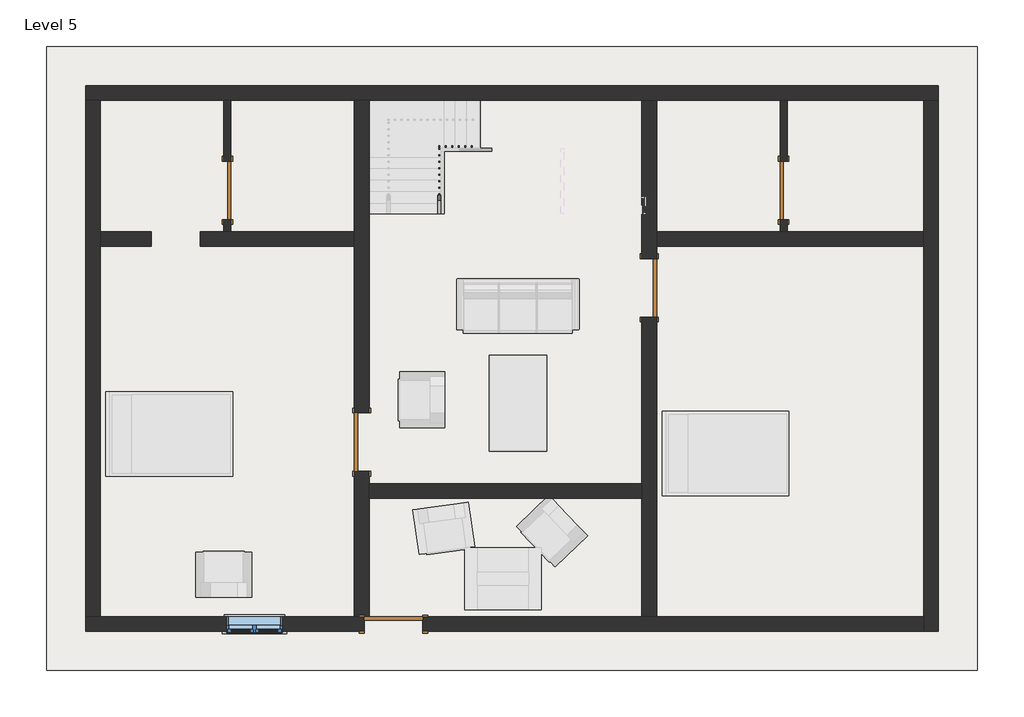
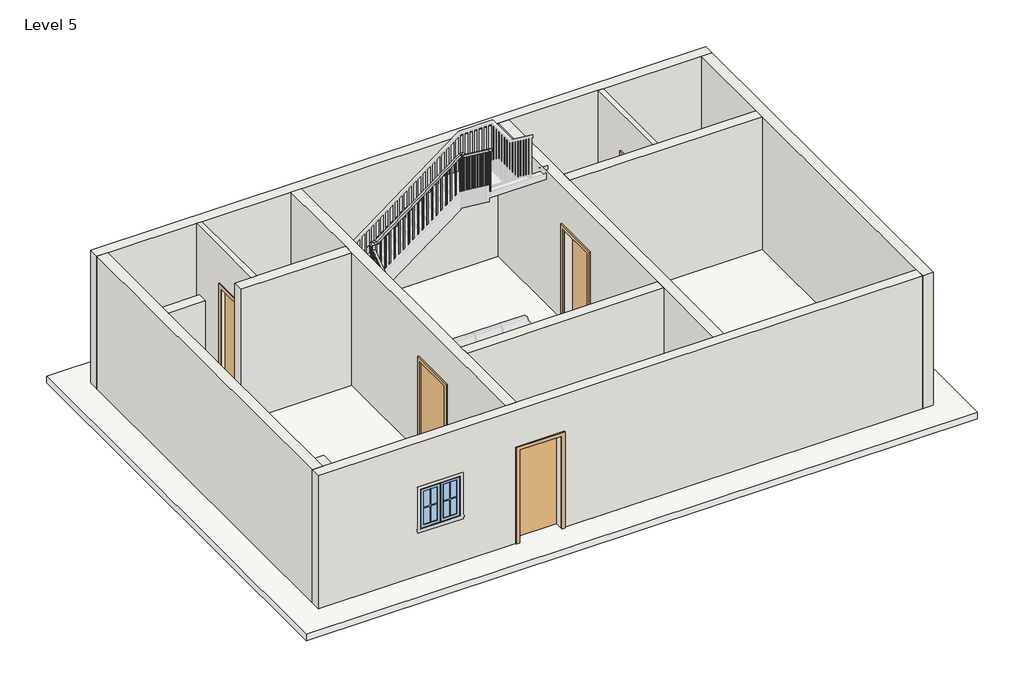
# One storey, part 1 of 2: 12 walls, 5 doors, 1 railing, 1 roof, 1 window.
"""IFC4 building model written with IfcOpenShell, lengths in millimetres."""

from ifc_helpers import new_model, si_unit, frame, origin, place, context, project, spatial, polyline, outline, extrude, faceted_brep, transform, mapped, element, save
from components import door_e5f9f3c4, door_a90ba1ad, door_305aa2a5, window_339605e1

model = new_model("IFC4")

# Units and contexts
model_context = context("Model", 3, world=origin())
ifc_project = project(units=[si_unit("LENGTHUNIT", "METRE", prefix="MILLI")], contexts=[model_context])

# Site, building, storey
site = spatial("IfcSite", under=ifc_project)
building = spatial("IfcBuilding", under=site)
storey = spatial("IfcBuildingStorey", under=building, Name="Level 5", Elevation=9601.2)

# Doors
placement = place(None, origin())
door_shape = door_e5f9f3c4(model_context)
element("IfcDoor", 1, ObjectType="Single-Flush : 36\" x 84\"", at=placement, inside=storey, context=model_context, shape_type="MappedRepresentation", body=[
    mapped(door_shape, transform((-5709.1546642, 5087.2167606, 9601.2), x_axis=(0.0, -1.0, 0.0), y_axis=(1.0, 0.0, 0.0), z_axis=(0.0, 0.0, 1.0))),
])
door_2_shape = door_a90ba1ad(model_context)
element("IfcDoor", 2, ObjectType="Single-Flush : 36\" x 84\"", at=placement, inside=storey, context=model_context, shape_type="MappedRepresentation", body=[
    mapped(door_2_shape, transform((-3607.3046642, 1150.2167606, 9601.2), x_axis=(0.0, -1.0, 0.0), y_axis=(1.0, 0.0, 0.0), z_axis=(0.0, 0.0, 1.0))),
])
element("IfcDoor", 3, ObjectType="Single-Flush : 36\" x 84\"", at=placement, inside=storey, context=model_context, shape_type="MappedRepresentation", body=[
    mapped(door_2_shape, transform((888.4953358, 3563.2167606, 9601.2), x_axis=(0.0, 1.0, 0.0), y_axis=(-1.0, 0.0, 0.0), z_axis=(0.0, 0.0, 1.0))),
])
element("IfcDoor", 4, ObjectType="Single-Flush : 36\" x 84\"", at=placement, inside=storey, context=model_context, shape_type="MappedRepresentation", body=[
    mapped(door_2_shape, transform((-3112.0046642, -1694.5832394, 9601.2), x_axis=(-1.0, 0.0, 0.0), y_axis=(0.0, -1.0, 0.0), z_axis=(0.0, 0.0, 1.0))),
])
door_3_shape = door_305aa2a5(model_context)
element("IfcDoor", 5, ObjectType="Single-Flush : 36\" x 84\"", at=placement, inside=storey, context=model_context, shape_type="MappedRepresentation", body=[
    mapped(door_3_shape, transform((2990.3453358, 5087.2167606, 9601.2), x_axis=(0.0, -1.0, 0.0), y_axis=(1.0, 0.0, 0.0), z_axis=(0.0, 0.0, 1.0))),
])

# Railing
element("IfcRailing", 6, ObjectType="Handrail - Rectangular", at=placement, inside=storey, context=model_context, shape_type="SolidModel", body=[
    faceted_brep([(-2419.4972892, 4718.9167606, 10648.1217391), (-2419.4972892, 4718.9167606, 10584.7634439), (-2368.6972892, 4718.9167606, 10584.7634439), (-2368.6972892, 4718.9167606, 10648.1217391), (-2419.4972892, 5670.3536537, 11357.2672495), (-2419.4972892, 5721.1536537, 11331.7723083), (-2368.6972892, 5721.1536537, 11331.7723083), (-2368.6972892, 5670.3536537, 11357.2672495), (-2419.4972892, 5670.3536537, 11464.0733611), (-2419.4972892, 5721.1536537, 11413.2733611), (-2368.6972892, 5721.1536537, 11413.2733611), (-2368.6972892, 5670.3536537, 11464.0733611), (-2419.4972892, 5797.3536537, 11464.0733611), (-2419.4972892, 5797.3536537, 11413.2733611), (-2368.6972892, 5746.5536537, 11413.2733611), (-2368.6972892, 5746.5536537, 11464.0733611), (-2292.4972892, 5797.3536537, 11464.0733611), (-2275.6482431, 5797.3536537, 11413.2733611), (-2275.6482431, 5746.5536537, 11413.2733611), (-2292.4972892, 5746.5536537, 11464.0733611), (-474.1369697, 5797.3536537, 12819.3729781), (-457.2879235, 5797.3536537, 12768.5729781), (-457.2879235, 5746.5536537, 12768.5729781), (-474.1369697, 5746.5536537, 12819.3729781), (-394.2046642, 5797.3536537, 12819.3729781), (-394.2046642, 5797.3536537, 12768.5729781), (-445.0046642, 5746.5536537, 12768.5729781), (-445.0046642, 5746.5536537, 12819.3729781), (-394.2046642, 5717.4213483, 12819.3729781), (-394.2046642, 5700.5723021, 12768.5729781), (-445.0046642, 5700.5723021, 12768.5729781), (-445.0046642, 5717.4213483, 12819.3729781), (-394.2046642, 4718.9167606, 13563.6), (-445.0046642, 4718.9167606, 13563.6), (-445.0046642, 4718.9167606, 13500.2417047), (-394.2046642, 4718.9167606, 13500.2417047)], [[[0, 1, 2, 3]], [[1, 0, 4, 5]], [[2, 1, 5, 6]], [[3, 2, 6, 7]], [[0, 3, 7, 4]], [[5, 4, 8, 9]], [[6, 5, 9, 10]], [[7, 6, 10, 11]], [[4, 7, 11, 8]], [[9, 8, 12, 13]], [[10, 9, 13, 14]], [[11, 10, 14, 15]], [[8, 11, 15, 12]], [[13, 12, 16, 17]], [[14, 13, 17, 18]], [[15, 14, 18, 19]], [[12, 15, 19, 16]], [[17, 16, 20, 21]], [[18, 17, 21, 22]], [[19, 18, 22, 23]], [[16, 19, 23, 20]], [[21, 20, 24, 25]], [[22, 21, 25, 26]], [[23, 22, 26, 27]], [[20, 23, 27, 24]], [[25, 24, 28, 29]], [[26, 25, 29, 30]], [[27, 26, 30, 31]], [[24, 27, 31, 28]], [[32, 33, 34, 35]], [[29, 28, 32, 35]], [[30, 29, 35, 34]], [[31, 30, 34, 33]], [[28, 31, 33, 32]]]),
    extrude(outline(polyline([(4746.4286537, 13479.7359459), (4765.4786537, 13465.5371882), (4765.4786537, 12516.6782609), (4746.4286537, 12516.6782609), (4746.4286537, 13479.7359459)])), frame((-429.1296642, 0.0, 0.0), z_axis=(1.0, 0.0, 0.0), x_axis=(0.0, 1.0, 0.0)), (0.0, 0.0, 1.0), 19.05),
    extrude(outline(polyline([(4848.0286537, 13404.0092378), (4867.0786537, 13389.8104801), (4867.0786537, 12516.6782609), (4848.0286537, 12516.6782609), (4848.0286537, 13404.0092378)])), frame((-429.1296642, 0.0, 0.0), z_axis=(1.0, 0.0, 0.0), x_axis=(0.0, 1.0, 0.0)), (0.0, 0.0, 1.0), 19.05),
    extrude(outline(polyline([(4949.6286537, 13328.2825298), (4968.6786537, 13314.083772), (4968.6786537, 12384.1565217), (4949.6286537, 12384.1565217), (4949.6286537, 13328.2825298)])), frame((-429.1296642, 0.0, 0.0), z_axis=(1.0, 0.0, 0.0), x_axis=(0.0, 1.0, 0.0)), (0.0, 0.0, 1.0), 19.05),
    extrude(outline(polyline([(5051.2286537, 13252.5558217), (5070.2786537, 13238.3570639), (5070.2786537, 12384.1565217), (5051.2286537, 12384.1565217), (5051.2286537, 13252.5558217)])), frame((-429.1296642, 0.0, 0.0), z_axis=(1.0, 0.0, 0.0), x_axis=(0.0, 1.0, 0.0)), (0.0, 0.0, 1.0), 19.05),
    extrude(outline(polyline([(5152.8286537, 13176.8291136), (5171.8786537, 13162.6303559), (5171.8786537, 12251.6347826), (5152.8286537, 12251.6347826), (5152.8286537, 13176.8291136)])), frame((-429.1296642, 0.0, 0.0), z_axis=(1.0, 0.0, 0.0), x_axis=(0.0, 1.0, 0.0)), (0.0, 0.0, 1.0), 19.05),
    extrude(outline(polyline([(5254.4286537, 13101.1024055), (5273.4786537, 13086.9036478), (5273.4786537, 12119.1130435), (5254.4286537, 12119.1130435), (5254.4286537, 13101.1024055)])), frame((-429.1296642, 0.0, 0.0), z_axis=(1.0, 0.0, 0.0), x_axis=(0.0, 1.0, 0.0)), (0.0, 0.0, 1.0), 19.05),
    extrude(outline(polyline([(5356.0286537, 13025.3756975), (5375.0786537, 13011.1769397), (5375.0786537, 12119.1130435), (5356.0286537, 12119.1130435), (5356.0286537, 13025.3756975)])), frame((-429.1296642, 0.0, 0.0), z_axis=(1.0, 0.0, 0.0), x_axis=(0.0, 1.0, 0.0)), (0.0, 0.0, 1.0), 19.05),
    extrude(outline(polyline([(5457.6286537, 12949.6489894), (5476.6786537, 12935.4502316), (5476.6786537, 11986.5913043), (5457.6286537, 11986.5913043), (5457.6286537, 12949.6489894)])), frame((-429.1296642, 0.0, 0.0), z_axis=(1.0, 0.0, 0.0), x_axis=(0.0, 1.0, 0.0)), (0.0, 0.0, 1.0), 19.05),
    extrude(outline(polyline([(5559.2286537, 12873.9222813), (5578.2786537, 12859.7235236), (5578.2786537, 11986.5913043), (5559.2286537, 11986.5913043), (5559.2286537, 12873.9222813)])), frame((-429.1296642, 0.0, 0.0), z_axis=(1.0, 0.0, 0.0), x_axis=(0.0, 1.0, 0.0)), (0.0, 0.0, 1.0), 19.05),
    extrude(outline(polyline([(5660.8286537, 12798.1955732), (5679.8786537, 12783.9968155), (5679.8786537, 11854.0695652), (5660.8286537, 11854.0695652), (5660.8286537, 12798.1955732)])), frame((-429.1296642, 0.0, 0.0), z_axis=(1.0, 0.0, 0.0), x_axis=(0.0, 1.0, 0.0)), (0.0, 0.0, 1.0), 19.05),
    extrude(outline(polyline([(-473.2222892, 5762.4286537), (-473.2222892, 5781.4786537), (-454.1722892, 5781.4786537), (-454.1722892, 5762.4286537), (-473.2222892, 5762.4286537)])), frame((0.0, 0.0, 11854.0695652), z_axis=(0.0, 0.0, 1.0), x_axis=(1.0, 0.0, 0.0)), (0.0, 0.0, 1.0), 914.5034129),
    extrude(outline(polyline([(12695.1684819, -555.7722892), (12680.9697242, -574.8222892), (11721.5478261, -574.8222892), (11721.5478261, -555.7722892), (12695.1684819, -555.7722892)])), frame((0.0, 5762.4286537, 0.0), z_axis=(0.0, 1.0, 0.0), x_axis=(0.0, 0.0, 1.0)), (0.0, 0.0, 1.0), 19.05),
    extrude(outline(polyline([(12619.4417739, -657.3722892), (12605.2430161, -676.4222892), (11721.5478261, -676.4222892), (11721.5478261, -657.3722892), (12619.4417739, -657.3722892)])), frame((0.0, 5762.4286537, 0.0), z_axis=(0.0, 1.0, 0.0), x_axis=(0.0, 0.0, 1.0)), (0.0, 0.0, 1.0), 19.05),
    extrude(outline(polyline([(12543.7150658, -758.9722892), (12529.516308, -778.0222892), (11589.026087, -778.0222892), (11589.026087, -758.9722892), (12543.7150658, -758.9722892)])), frame((0.0, 5762.4286537, 0.0), z_axis=(0.0, 1.0, 0.0), x_axis=(0.0, 0.0, 1.0)), (0.0, 0.0, 1.0), 19.05),
    extrude(outline(polyline([(12467.9883577, -860.5722892), (12453.7896, -879.6222892), (11589.026087, -879.6222892), (11589.026087, -860.5722892), (12467.9883577, -860.5722892)])), frame((0.0, 5762.4286537, 0.0), z_axis=(0.0, 1.0, 0.0), x_axis=(0.0, 0.0, 1.0)), (0.0, 0.0, 1.0), 19.05),
    extrude(outline(polyline([(12392.2616496, -962.1722892), (12378.0628919, -981.2222892), (11456.5043478, -981.2222892), (11456.5043478, -962.1722892), (12392.2616496, -962.1722892)])), frame((0.0, 5762.4286537, 0.0), z_axis=(0.0, 1.0, 0.0), x_axis=(0.0, 0.0, 1.0)), (0.0, 0.0, 1.0), 19.05),
    extrude(outline(polyline([(12316.5349416, -1063.7722892), (12302.3361838, -1082.8222892), (11456.5043478, -1082.8222892), (11456.5043478, -1063.7722892), (12316.5349416, -1063.7722892)])), frame((0.0, 5762.4286537, 0.0), z_axis=(0.0, 1.0, 0.0), x_axis=(0.0, 0.0, 1.0)), (0.0, 0.0, 1.0), 19.05),
    extrude(outline(polyline([(12240.8082335, -1165.3722892), (12226.6094757, -1184.4222892), (11323.9826087, -1184.4222892), (11323.9826087, -1165.3722892), (12240.8082335, -1165.3722892)])), frame((0.0, 5762.4286537, 0.0), z_axis=(0.0, 1.0, 0.0), x_axis=(0.0, 0.0, 1.0)), (0.0, 0.0, 1.0), 19.05),
    extrude(outline(polyline([(12165.0815254, -1266.9722892), (12150.8827677, -1286.0222892), (11191.4608696, -1286.0222892), (11191.4608696, -1266.9722892), (12165.0815254, -1266.9722892)])), frame((0.0, 5762.4286537, 0.0), z_axis=(0.0, 1.0, 0.0), x_axis=(0.0, 0.0, 1.0)), (0.0, 0.0, 1.0), 19.05),
    extrude(outline(polyline([(12089.3548173, -1368.5722892), (12075.1560596, -1387.6222892), (11191.4608696, -1387.6222892), (11191.4608696, -1368.5722892), (12089.3548173, -1368.5722892)])), frame((0.0, 5762.4286537, 0.0), z_axis=(0.0, 1.0, 0.0), x_axis=(0.0, 0.0, 1.0)), (0.0, 0.0, 1.0), 19.05),
    extrude(outline(polyline([(12013.6281093, -1470.1722892), (11999.4293515, -1489.2222892), (11058.9391304, -1489.2222892), (11058.9391304, -1470.1722892), (12013.6281093, -1470.1722892)])), frame((0.0, 5762.4286537, 0.0), z_axis=(0.0, 1.0, 0.0), x_axis=(0.0, 0.0, 1.0)), (0.0, 0.0, 1.0), 19.05),
    extrude(outline(polyline([(11937.9014012, -1571.7722892), (11923.7026434, -1590.8222892), (11058.9391304, -1590.8222892), (11058.9391304, -1571.7722892), (11937.9014012, -1571.7722892)])), frame((0.0, 5762.4286537, 0.0), z_axis=(0.0, 1.0, 0.0), x_axis=(0.0, 0.0, 1.0)), (0.0, 0.0, 1.0), 19.05),
    extrude(outline(polyline([(11862.1746931, -1673.3722892), (11847.9759354, -1692.4222892), (10926.4173913, -1692.4222892), (10926.4173913, -1673.3722892), (11862.1746931, -1673.3722892)])), frame((0.0, 5762.4286537, 0.0), z_axis=(0.0, 1.0, 0.0), x_axis=(0.0, 0.0, 1.0)), (0.0, 0.0, 1.0), 19.05),
    extrude(outline(polyline([(11786.447985, -1774.9722892), (11772.2492273, -1794.0222892), (10926.4173913, -1794.0222892), (10926.4173913, -1774.9722892), (11786.447985, -1774.9722892)])), frame((0.0, 5762.4286537, 0.0), z_axis=(0.0, 1.0, 0.0), x_axis=(0.0, 0.0, 1.0)), (0.0, 0.0, 1.0), 19.05),
    extrude(outline(polyline([(11710.721277, -1876.5722892), (11696.5225192, -1895.6222892), (10793.8956522, -1895.6222892), (10793.8956522, -1876.5722892), (11710.721277, -1876.5722892)])), frame((0.0, 5762.4286537, 0.0), z_axis=(0.0, 1.0, 0.0), x_axis=(0.0, 0.0, 1.0)), (0.0, 0.0, 1.0), 19.05),
    extrude(outline(polyline([(11634.9945689, -1978.1722892), (11620.7958111, -1997.2222892), (10661.373913, -1997.2222892), (10661.373913, -1978.1722892), (11634.9945689, -1978.1722892)])), frame((0.0, 5762.4286537, 0.0), z_axis=(0.0, 1.0, 0.0), x_axis=(0.0, 0.0, 1.0)), (0.0, 0.0, 1.0), 19.05),
    extrude(outline(polyline([(11559.2678608, -2079.7722892), (11545.0691031, -2098.8222892), (10661.373913, -2098.8222892), (10661.373913, -2079.7722892), (11559.2678608, -2079.7722892)])), frame((0.0, 5762.4286537, 0.0), z_axis=(0.0, 1.0, 0.0), x_axis=(0.0, 0.0, 1.0)), (0.0, 0.0, 1.0), 19.05),
    extrude(outline(polyline([(11483.5411527, -2181.3722892), (11469.342395, -2200.4222892), (10528.8521739, -2200.4222892), (10528.8521739, -2181.3722892), (11483.5411527, -2181.3722892)])), frame((0.0, 5762.4286537, 0.0), z_axis=(0.0, 1.0, 0.0), x_axis=(0.0, 0.0, 1.0)), (0.0, 0.0, 1.0), 19.05),
    extrude(outline(polyline([(11407.8144447, -2282.9722892), (11393.6156869, -2302.0222892), (10528.8521739, -2302.0222892), (10528.8521739, -2282.9722892), (11407.8144447, -2282.9722892)])), frame((0.0, 5762.4286537, 0.0), z_axis=(0.0, 1.0, 0.0), x_axis=(0.0, 0.0, 1.0)), (0.0, 0.0, 1.0), 19.05),
    extrude(outline(polyline([(-2384.5722892, 5725.3917606), (-2403.6222892, 5725.3917606), (-2403.6222892, 5744.4417606), (-2384.5722892, 5744.4417606), (-2384.5722892, 5725.3917606)])), frame((0.0, 0.0, 10396.3304348), z_axis=(0.0, 0.0, 1.0), x_axis=(1.0, 0.0, 0.0)), (0.0, 0.0, 1.0), 1016.9429263),
    extrude(outline(polyline([(5623.7917606, 11259.2044377), (5642.8417606, 11273.4031954), (5642.8417606, 10396.3304348), (5623.7917606, 10396.3304348), (5623.7917606, 11259.2044377)])), frame((-2403.6222892, 0.0, 0.0), z_axis=(1.0, 0.0, 0.0), x_axis=(0.0, 1.0, 0.0)), (0.0, 0.0, 1.0), 19.05),
    extrude(outline(polyline([(5522.1917606, 11183.4777296), (5541.2417606, 11197.6764873), (5541.2417606, 10263.8086957), (5522.1917606, 10263.8086957), (5522.1917606, 11183.4777296)])), frame((-2403.6222892, 0.0, 0.0), z_axis=(1.0, 0.0, 0.0), x_axis=(0.0, 1.0, 0.0)), (0.0, 0.0, 1.0), 19.05),
    extrude(outline(polyline([(5420.5917606, 11107.7510215), (5439.6417606, 11121.9497793), (5439.6417606, 10263.8086957), (5420.5917606, 10263.8086957), (5420.5917606, 11107.7510215)])), frame((-2403.6222892, 0.0, 0.0), z_axis=(1.0, 0.0, 0.0), x_axis=(0.0, 1.0, 0.0)), (0.0, 0.0, 1.0), 19.05),
    extrude(outline(polyline([(5318.9917606, 11032.0243134), (5338.0417606, 11046.2230712), (5338.0417606, 10131.2869565), (5318.9917606, 10131.2869565), (5318.9917606, 11032.0243134)])), frame((-2403.6222892, 0.0, 0.0), z_axis=(1.0, 0.0, 0.0), x_axis=(0.0, 1.0, 0.0)), (0.0, 0.0, 1.0), 19.05),
    extrude(outline(polyline([(5217.3917606, 10956.2976054), (5236.4417606, 10970.4963631), (5236.4417606, 9998.7652174), (5217.3917606, 9998.7652174), (5217.3917606, 10956.2976054)])), frame((-2403.6222892, 0.0, 0.0), z_axis=(1.0, 0.0, 0.0), x_axis=(0.0, 1.0, 0.0)), (0.0, 0.0, 1.0), 19.05),
    extrude(outline(polyline([(5115.7917606, 10880.5708973), (5134.8417606, 10894.769655), (5134.8417606, 9998.7652174), (5115.7917606, 9998.7652174), (5115.7917606, 10880.5708973)])), frame((-2403.6222892, 0.0, 0.0), z_axis=(1.0, 0.0, 0.0), x_axis=(0.0, 1.0, 0.0)), (0.0, 0.0, 1.0), 19.05),
    extrude(outline(polyline([(5014.1917606, 10804.8441892), (5033.2417606, 10819.042947), (5033.2417606, 9866.2434783), (5014.1917606, 9866.2434783), (5014.1917606, 10804.8441892)])), frame((-2403.6222892, 0.0, 0.0), z_axis=(1.0, 0.0, 0.0), x_axis=(0.0, 1.0, 0.0)), (0.0, 0.0, 1.0), 19.05),
    extrude(outline(polyline([(4912.5917606, 10729.1174811), (4931.6417606, 10743.3162389), (4931.6417606, 9866.2434783), (4912.5917606, 9866.2434783), (4912.5917606, 10729.1174811)])), frame((-2403.6222892, 0.0, 0.0), z_axis=(1.0, 0.0, 0.0), x_axis=(0.0, 1.0, 0.0)), (0.0, 0.0, 1.0), 19.05),
    extrude(outline(polyline([(4810.9917606, 10653.3907731), (4830.0417606, 10667.5895308), (4830.0417606, 9733.7217391), (4810.9917606, 9733.7217391), (4810.9917606, 10653.3907731)])), frame((-2403.6222892, 0.0, 0.0), z_axis=(1.0, 0.0, 0.0), x_axis=(0.0, 1.0, 0.0)), (0.0, 0.0, 1.0), 19.05),
    extrude(outline(polyline([(-429.1296642, 5762.4286537), (-429.1296642, 5781.4786537), (-410.0796642, 5781.4786537), (-410.0796642, 5762.4286537), (-429.1296642, 5762.4286537)])), frame((0.0, 0.0, 11854.0695652), z_axis=(0.0, 0.0, 1.0), x_axis=(1.0, 0.0, 0.0)), (0.0, 0.0, 1.0), 914.5034129),
    extrude(outline(polyline([(-2384.5722892, 5762.4286537), (-2403.6222892, 5762.4286537), (-2403.6222892, 5781.4786537), (-2384.5722892, 5781.4786537), (-2384.5722892, 5762.4286537)])), frame((0.0, 0.0, 10396.3304348), z_axis=(0.0, 0.0, 1.0), x_axis=(1.0, 0.0, 0.0)), (0.0, 0.0, 1.0), 1016.9429263),
    extrude(outline(polyline([(4718.9167606, 13500.2417047), (4737.9667606, 13486.042947), (4737.9667606, 12516.6782609), (4718.9167606, 12516.6782609), (4718.9167606, 13500.2417047)])), frame((-429.1296642, 0.0, 0.0), z_axis=(1.0, 0.0, 0.0), x_axis=(0.0, 1.0, 0.0)), (0.0, 0.0, 1.0), 19.05),
    extrude(outline(polyline([(4718.9167606, 10584.7634439), (4737.9667606, 10598.9622016), (4737.9667606, 9733.7217391), (4718.9167606, 9733.7217391), (4718.9167606, 10584.7634439)])), frame((-2403.6222892, 0.0, 0.0), z_axis=(1.0, 0.0, 0.0), x_axis=(0.0, 1.0, 0.0)), (0.0, 0.0, 1.0), 19.05),
])

# Roof
element("IfcRoof", 7, ObjectType="Generic - 12\"", at=placement, inside=storey, context=model_context, shape_type="SweptSolid", body=[
    extrude(outline(polyline([(-8534.9046642, 7335.1167606), (6019.2953358, 7335.1167606), (6019.2953358, -2418.4832394), (-8534.9046642, -2418.4832394), (-8534.9046642, 7335.1167606)])), frame((0.0, 0.0, 9448.8), z_axis=(0.0, 0.0, 1.0), x_axis=(1.0, 0.0, 0.0)), (0.0, 0.0, 1.0), 152.4),
])

# Walls
element("IfcWall", 8, ObjectType="WALL4.5\"", at=placement, inside=storey, context=model_context, shape_type="SweptSolid", body=[
    extrude(outline(polyline([(4630.0167606, 11734.8), (4630.0167606, 9601.2), (4439.5167606, 9601.2), (4439.5167606, 12649.2), (6496.9167606, 12649.2), (6496.9167606, 9601.2), (5544.4167606, 9601.2), (5544.4167606, 11734.8), (4630.0167606, 11734.8)])), frame((-5766.3046642, 0.0, 0.0), z_axis=(1.0, 0.0, 0.0), x_axis=(0.0, 1.0, 0.0)), (0.0, 0.0, 1.0), 114.3),
])
element("IfcWall", 9, ObjectType="WALL4.5\"", at=placement, inside=storey, context=model_context, shape_type="SweptSolid", body=[
    extrude(outline(polyline([(4630.0167606, 11734.8), (4630.0167606, 9601.2), (4439.5167606, 9601.2), (4439.5167606, 12649.2), (6496.9167606, 12649.2), (6496.9167606, 9601.2), (5544.4167606, 9601.2), (5544.4167606, 11734.8), (4630.0167606, 11734.8)])), frame((2933.1953358, 0.0, 0.0), z_axis=(1.0, 0.0, 0.0), x_axis=(0.0, 1.0, 0.0)), (0.0, 0.0, 1.0), 114.3),
])
element("IfcWall", 10, ObjectType="WALL9\"", at=placement, inside=storey, context=model_context, shape_type="Brep", body=[
    faceted_brep([(-7925.3046642, 6496.9167606, 9601.2), (-7696.7046642, 6496.9167606, 9601.2), (-5766.3046642, 6496.9167606, 9601.2), (-5652.0046642, 6496.9167606, 9601.2), (-3721.6046642, 6496.9167606, 9601.2), (-3493.0046642, 6496.9167606, 9601.2), (774.1953358, 6496.9167606, 9601.2), (1002.7953358, 6496.9167606, 9601.2), (2933.1953358, 6496.9167606, 9601.2), (3047.4953358, 6496.9167606, 9601.2), (5181.0953358, 6496.9167606, 9601.2), (5409.6953358, 6496.9167606, 9601.2), (5409.6953358, 6496.9167606, 12649.2), (5181.0953358, 6496.9167606, 12649.2), (3047.4953358, 6496.9167606, 12649.2), (2933.1953358, 6496.9167606, 12649.2), (1002.7953358, 6496.9167606, 12649.2), (774.1953358, 6496.9167606, 12649.2), (-3493.0046642, 6496.9167606, 12649.2), (-3721.6046642, 6496.9167606, 12649.2), (-5652.0046642, 6496.9167606, 12649.2), (-5766.3046642, 6496.9167606, 12649.2), (-7696.7046642, 6496.9167606, 12649.2), (-7925.3046642, 6496.9167606, 12649.2), (-7925.3046642, 6725.5167606, 9601.2), (-7925.3046642, 6725.5167606, 12649.2), (5409.6953358, 6725.5167606, 12649.2), (5409.6953358, 6725.5167606, 9601.2)], [[[0, 1, 2, 3, 4, 5, 6, 7, 8, 9, 10, 11, 12, 13, 14, 15, 16, 17, 18, 19, 20, 21, 22, 23]], [[24, 25, 26, 27]], [[11, 10, 9, 8, 7, 6, 5, 4, 3, 2, 1, 0, 24, 27]], [[12, 11, 27, 26]], [[0, 23, 25, 24]], [[23, 22, 21, 20, 19, 18, 17, 16, 15, 14, 13, 12, 26, 25]]]),
])
element("IfcWall", 11, ObjectType="WALL9\"", at=placement, inside=storey, context=model_context, shape_type="Brep", body=[
    faceted_brep([(5181.0953358, 6496.9167606, 9601.2), (5181.0953358, 4439.5167606, 9601.2), (5181.0953358, 4210.9167606, 9601.2), (5181.0953358, -1580.2832394, 9601.2), (5181.0953358, -1808.8832394, 9601.2), (5181.0953358, -1808.8832394, 12649.2), (5181.0953358, -1580.2832394, 12649.2), (5181.0953358, 4210.9167606, 12649.2), (5181.0953358, 4439.5167606, 12649.2), (5181.0953358, 6496.9167606, 12649.2), (5409.6953358, 6496.9167606, 9601.2), (5409.6953358, 6496.9167606, 12649.2), (5409.6953358, -1808.8832394, 12649.2), (5409.6953358, -1808.8832394, 9601.2)], [[[0, 1, 2, 3, 4, 5, 6, 7, 8, 9]], [[10, 11, 12, 13]], [[4, 3, 2, 1, 0, 10, 13]], [[0, 9, 11, 10]], [[5, 4, 13, 12]], [[9, 8, 7, 6, 5, 12, 11]]]),
])
element("IfcWall", 12, ObjectType="WALL9\"", at=placement, inside=storey, context=model_context, shape_type="Brep", body=[
    faceted_brep([(-3569.2046642, -1580.2832394, 11734.8), (-3569.2046642, -1580.2832394, 9601.2), (-3721.6046642, -1580.2832394, 9601.2), (-7696.7046642, -1580.2832394, 9601.2), (-7925.3046642, -1580.2832394, 9601.2), (-7925.3046642, -1580.2832394, 12649.2), (-7696.7046642, -1580.2832394, 12649.2), (-3721.6046642, -1580.2832394, 12649.2), (-3493.0046642, -1580.2832394, 12649.2), (774.1953358, -1580.2832394, 12649.2), (1002.7953358, -1580.2832394, 12649.2), (5181.0953358, -1580.2832394, 12649.2), (5181.0953358, -1580.2832394, 9601.2), (1002.7953358, -1580.2832394, 9601.2), (774.1953358, -1580.2832394, 9601.2), (-2654.8046642, -1580.2832394, 9601.2), (-2654.8046642, -1580.2832394, 11734.8), (-5715.5046642, -1580.2832394, 11582.7434313), (-5715.5046642, -1580.2832394, 10668.3434313), (-4851.9046642, -1580.2832394, 10668.3434313), (-4851.9046642, -1580.2832394, 11582.7434313), (-7925.3046642, -1808.8832394, 9601.2), (-3569.2046642, -1808.8832394, 9601.2), (-3569.2046642, -1808.8832394, 11734.8), (-2654.8046642, -1808.8832394, 11734.8), (-2654.8046642, -1808.8832394, 9601.2), (5181.0953358, -1808.8832394, 9601.2), (5181.0953358, -1808.8832394, 12649.2), (-7925.3046642, -1808.8832394, 12649.2), (-5715.5046642, -1808.8832394, 11582.7434313), (-4851.9046642, -1808.8832394, 11582.7434313), (-4851.9046642, -1808.8832394, 10668.3434313), (-5715.5046642, -1808.8832394, 10668.3434313)], [[[0, 1, 2, 3, 4, 5, 6, 7, 8, 9, 10, 11, 12, 13, 14, 15, 16], [17, 18, 19, 20]], [[21, 22, 23, 24, 25, 26, 27, 28], [29, 30, 31, 32]], [[4, 3, 2, 1, 22, 21]], [[15, 14, 13, 12, 26, 25]], [[12, 11, 27, 26]], [[5, 4, 21, 28]], [[23, 22, 1, 0]], [[24, 23, 0, 16]], [[25, 24, 16, 15]], [[11, 10, 9, 8, 7, 6, 5, 28, 27]], [[18, 17, 29, 32]], [[19, 18, 32, 31]], [[20, 19, 31, 30]], [[17, 20, 30, 29]]]),
])
element("IfcWall", 13, ObjectType="WALL9\"", at=placement, inside=storey, context=model_context, shape_type="Brep", body=[
    faceted_brep([(-7696.7046642, -1580.2832394, 9601.2), (-7696.7046642, 4210.9167606, 9601.2), (-7696.7046642, 4439.5167606, 9601.2), (-7696.7046642, 6496.9167606, 9601.2), (-7696.7046642, 6496.9167606, 12649.2), (-7696.7046642, 4439.5167606, 12649.2), (-7696.7046642, 4210.9167606, 12649.2), (-7696.7046642, -1580.2832394, 12649.2), (-7925.3046642, -1580.2832394, 9601.2), (-7925.3046642, -1580.2832394, 12649.2), (-7925.3046642, 6496.9167606, 12649.2), (-7925.3046642, 6496.9167606, 9601.2)], [[[0, 1, 2, 3, 4, 5, 6, 7]], [[8, 9, 10, 11]], [[3, 2, 1, 0, 8, 11]], [[4, 3, 11, 10]], [[0, 7, 9, 8]], [[7, 6, 5, 4, 10, 9]]]),
])
element("IfcWall", 14, ObjectType="WALL9\"", at=placement, inside=storey, context=model_context, shape_type="Brep", body=[
    faceted_brep([(-3721.6046642, 693.0167606, 11734.8), (-3721.6046642, 693.0167606, 9601.2), (-3721.6046642, -1580.2832394, 9601.2), (-3721.6046642, -1580.2832394, 12649.2), (-3721.6046642, 4210.9167606, 12649.2), (-3721.6046642, 4439.5167606, 12649.2), (-3721.6046642, 6496.9167606, 12649.2), (-3721.6046642, 6496.9167606, 9601.2), (-3721.6046642, 4439.5167606, 9601.2), (-3721.6046642, 4210.9167606, 9601.2), (-3721.6046642, 1607.4167606, 9601.2), (-3721.6046642, 1607.4167606, 11734.8), (-3493.0046642, -1580.2832394, 9601.2), (-3493.0046642, 273.9167606, 9601.2), (-3493.0046642, 502.5167606, 9601.2), (-3493.0046642, 693.0167606, 9601.2), (-3493.0046642, 693.0167606, 11734.8), (-3493.0046642, 1607.4167606, 11734.8), (-3493.0046642, 1607.4167606, 9601.2), (-3493.0046642, 6496.9167606, 9601.2), (-3493.0046642, 6496.9167606, 12649.2), (-3493.0046642, 4718.9167606, 12649.2), (-3493.0046642, 502.5167606, 12649.2), (-3493.0046642, 273.9167606, 12649.2), (-3493.0046642, -1580.2832394, 12649.2), (-3569.2046642, -1580.2832394, 9601.2)], [[[0, 1, 2, 3, 4, 5, 6, 7, 8, 9, 10, 11]], [[12, 13, 14, 15, 16, 17, 18, 19, 20, 21, 22, 23, 24]], [[2, 1, 15, 14, 13, 12, 25]], [[10, 9, 8, 7, 19, 18]], [[7, 6, 20, 19]], [[3, 2, 25, 12, 24]], [[16, 15, 1, 0]], [[17, 16, 0, 11]], [[18, 17, 11, 10]], [[6, 5, 4, 3, 24, 23, 22, 21, 20]]]),
])
element("IfcWall", 15, ObjectType="WALL9\"", at=placement, inside=storey, context=model_context, shape_type="Brep", body=[
    faceted_brep([(774.1953358, 6496.9167606, 9601.2), (774.1953358, 4020.4167606, 9601.2), (774.1953358, 4020.4167606, 11734.8), (774.1953358, 3106.0167606, 11734.8), (774.1953358, 3106.0167606, 9601.2), (774.1953358, 502.5167606, 9601.2), (774.1953358, 273.9167606, 9601.2), (774.1953358, -1580.2832394, 9601.2), (774.1953358, -1580.2832394, 12649.2), (774.1953358, 273.9167606, 12649.2), (774.1953358, 502.5167606, 12649.2), (774.1953358, 4718.9167606, 12649.2), (774.1953358, 6496.9167606, 12649.2), (1002.7953358, 4020.4167606, 11734.8), (1002.7953358, 4020.4167606, 9601.2), (1002.7953358, 4210.9167606, 9601.2), (1002.7953358, 4439.5167606, 9601.2), (1002.7953358, 6496.9167606, 9601.2), (1002.7953358, 6496.9167606, 12649.2), (1002.7953358, 4439.5167606, 12649.2), (1002.7953358, 4210.9167606, 12649.2), (1002.7953358, -1580.2832394, 12649.2), (1002.7953358, -1580.2832394, 9601.2), (1002.7953358, 3106.0167606, 9601.2), (1002.7953358, 3106.0167606, 11734.8)], [[[0, 1, 2, 3, 4, 5, 6, 7, 8, 9, 10, 11, 12]], [[13, 14, 15, 16, 17, 18, 19, 20, 21, 22, 23, 24]], [[23, 22, 7, 6, 5, 4]], [[17, 16, 15, 14, 1, 0]], [[0, 12, 18, 17]], [[8, 7, 22, 21]], [[2, 1, 14, 13]], [[3, 2, 13, 24]], [[4, 3, 24, 23]], [[12, 11, 10, 9, 8, 21, 20, 19, 18]]]),
])
element("IfcWall", 16, ObjectType="WALL9\"", at=placement, inside=storey, context=model_context, shape_type="SweptSolid", body=[
    extrude(outline(polyline([(774.1953358, 273.9167606), (-3493.0046642, 273.9167606), (-3493.0046642, 502.5167606), (774.1953358, 502.5167606), (774.1953358, 273.9167606)])), frame((0.0, 0.0, 9601.2), z_axis=(0.0, 0.0, 1.0), x_axis=(1.0, 0.0, 0.0)), (0.0, 0.0, 1.0), 3048.0),
])
element("IfcWall", 17, ObjectType="WALL9\"", at=placement, inside=storey, context=model_context, shape_type="SweptSolid", body=[
    extrude(outline(polyline([(-6895.4507894, 4210.9167606), (-7696.7046642, 4210.9167606), (-7696.7046642, 4439.5167606), (-6895.4507894, 4439.5167606), (-6895.4507894, 4210.9167606)])), frame((0.0, 0.0, 9601.2), z_axis=(0.0, 0.0, 1.0), x_axis=(1.0, 0.0, 0.0)), (0.0, 0.0, 1.0), 3048.0),
])
element("IfcWall", 18, ObjectType="WALL9\"", at=placement, inside=storey, context=model_context, shape_type="Brep", body=[
    faceted_brep([(-3721.6046642, 4439.5167606, 9601.2), (-5652.0046642, 4439.5167606, 9601.2), (-5766.3046642, 4439.5167606, 9601.2), (-6131.0963491, 4439.5167606, 9601.2), (-6131.0963491, 4439.5167606, 12649.2), (-5766.3046642, 4439.5167606, 12649.2), (-5652.0046642, 4439.5167606, 12649.2), (-3721.6046642, 4439.5167606, 12649.2), (-3721.6046642, 4210.9167606, 9601.2), (-3721.6046642, 4210.9167606, 12649.2), (-6131.0963491, 4210.9167606, 12649.2), (-6131.0963491, 4210.9167606, 9601.2)], [[[0, 1, 2, 3, 4, 5, 6, 7]], [[8, 9, 10, 11]], [[3, 2, 1, 0, 8, 11]], [[4, 3, 11, 10]], [[0, 7, 9, 8]], [[7, 6, 5, 4, 10, 9]]]),
])
element("IfcWall", 19, ObjectType="WALL9\"", at=placement, inside=storey, context=model_context, shape_type="Brep", body=[
    faceted_brep([(1002.7953358, 4210.9167606, 9601.2), (5181.0953358, 4210.9167606, 9601.2), (5181.0953358, 4210.9167606, 12649.2), (1002.7953358, 4210.9167606, 12649.2), (1002.7953358, 4439.5167606, 9601.2), (1002.7953358, 4439.5167606, 12649.2), (2933.1953358, 4439.5167606, 12649.2), (3047.4953358, 4439.5167606, 12649.2), (5181.0953358, 4439.5167606, 12649.2), (5181.0953358, 4439.5167606, 9601.2), (3047.4953358, 4439.5167606, 9601.2), (2933.1953358, 4439.5167606, 9601.2)], [[[0, 1, 2, 3]], [[4, 5, 6, 7, 8, 9, 10, 11]], [[1, 0, 4, 11, 10, 9]], [[2, 1, 9, 8]], [[0, 3, 5, 4]], [[3, 2, 8, 7, 6, 5]]]),
])

# Window
window_shape = window_339605e1(model_context)
element("IfcWindow", 20, ObjectType="Window-Casement-Double : 34\" x 36\"", at=placement, inside=storey, context=model_context, shape_type="MappedRepresentation", body=[
    mapped(window_shape, transform((-5283.7046642, -1694.5832394, 9753.9434313), x_axis=(-1.0, 0.0, 0.0), y_axis=(0.0, -1.0, 0.0), z_axis=(0.0, 0.0, 1.0))),
])

save(model, "model.ifc")

# Revit data of these elements
# Type "Single-Flush : 36\" x 84\""
#   Type Mark = "1"
#   Construction Type Id = "MDOOR"
#   Assembly Code = "C1020"
#   Analytic Construction = "Metal"
#   Thickness = 0' - 2"
#   Heat Transfer Coefficient (U) = 0.651978 BTU/(h·ft²·°F)
#   Height = 7' - 0"
#   Trim Projection Ext = 0' - 1"
#   Trim Projection Int = 0' - 1"
#   Trim Width = 0' - 3"
#   Width = 3' - 0"
#   Define Thermal Properties by = 1
#   Define Thermal Properties by = 1
#   Door Material = Door - Panel
#   Frame Material = Door - Frame
#   Visual Light Transmittance = 0
#   Solar Heat Gain Coefficient = 0
#   Function = (empty or 0)
#   Wall Closure = (empty or 0)
# Type "Handrail - Rectangular"
#   Assembly Code = "C2010400"
#   built-in parameter 1008612 = 0.0416667 (stored number, unit not read)
#   built-in parameter 1008611 = 0.0416667 (stored number, unit not read)
#   built-in parameter 1008609 = 0.333333 (stored number, unit not read)
#   built-in parameter 1008604 = 0.166667 (stored number, unit not read)
#   built-in parameter 1008603 = 0.166667 (stored number, unit not read)
#   Railing Height = 3' - 0"
#   built-in parameter 1008630 = 2
#   built-in parameter 1008610 = 2
#   built-in parameter 1008618 = Baluster - Square : 3/4"
# Type "Generic - 12\""
#   Assembly Code = "B1020"
#   Layers, outside or top first: 0' - 6" no material (function 1)
# Type "WALL4.5\""
#   Assembly Code = "B2010"
#   Layers, outside or top first: 0' - 4 1/2" no material (function 1)
# Type "WALL9\""
#   Assembly Code = "B2010"
#   Layers, outside or top first: 0' - 9" no material (function 1)
# Type "Window-Casement-Double : 34\" x 36\""
#   Type Mark = "14"
#   Fire Rating = "0.5h"
#   Assembly Code = "B2020100"
#   Analytic Construction = "Double glazing - domestic"
#   Frame Extension [instance default] = 0' - 0 1/4"
#   Window Inset [instance default] = 0' - 0"
#   Wall Thickness [instance default] = 0' - 6"
#   Interior Wall Closure [instance default] = 0' - 2 1/4"
#   Half Width = 1' - 5"
#   Visual Light Transmittance = 0.81
#   Thermal Resistance (R) = 1.8146 (h·ft²·°F)/BTU
#   Solar Heat Gain Coefficient = 0.76
#   Rough Width = 2' - 10 1/2"
#   Rough Height = 3' - 0 1/2"
#   Height = 3' - 0"
#   Heat Transfer Coefficient (U) = 0.5511 BTU/(h·ft²·°F)
#   Exterior Wall Closure [instance default] = 0' - 1 1/4"
#   Extension Jamb [instance default] = 0' - 2 1/4"
#   Default Sill Height = 3' - 0"
#   Width = 2' - 10"
#   Define Thermal Properties by = 0
#   Muntin Visibility = yes
#   Interior Trim Visibility [instance default] = yes
#   Exterior Trim Visibility [instance default] = yes
#   Extension Jamb Visibility [instance default] = yes
#   Interior Trim Material = Wood - Stained
#   Muntin Pattern = Muntin Pattern_2x2 : Muntin Pattern_2x2
#   Interior Trim = Trim-Window-Interior-Flat : Picture Frame
#   Interior Frame Material = Wood - Stained
#   Glass Panel Material = Glass
#   Exterior Trim Material = Clad - White
#   Exterior Trim = Trim-Window-Exterior-Flat : with Sill
#   Exterior Frame Material = Clad - White
#   Wall Closure = (empty or 0)
# Elements 1, 2, 3, 4, 5 (IfcDoor, "Single-Flush : 36\" x 84\"")
#   Phase Created = New Construction
#   Materials on its faces: "Door - Frame", "Door - Panel"
# Element 6 (IfcRailing, "Handrail - Rectangular")
#   Phase Created = New Construction
# Element 7 (IfcRoof, "Generic - 12\"")
#   built-in parameter 1001705 = 31.5 (stored number, unit not read)
#   built-in parameter 1001701 = -0.5 (stored number, unit not read)
#   built-in parameter 1001710 = 33615
#   Phase Created = New Construction
#   Materials on its faces: "Default Roof"
# Elements 8, 9 (IfcWall, "WALL4.5\"")
#   Top Offset = 0' - 0"
#   Base Offset = 0' - 0"
#   Unconnected Height = 10' - 0"
#   wall height = 10' - 0"
#   Phase Created = New Construction
#   Base Constraint = Level 5
#   Materials on its faces: "Default Wall"
# Elements 10, 11, 12, 13, 14, 15, 16, 17, 18, 19 (IfcWall, "WALL9\"")
#   Top Offset = 0' - 0"
#   Base Offset = 0' - 0"
#   Unconnected Height = 10' - 0"
#   wall height = 10' - 0"
#   Phase Created = New Construction
#   Base Constraint = Level 5
#   Materials on its faces: "Default Wall"
# Element 20 (IfcWindow, "Window-Casement-Double : 34\" x 36\"")
#   Mark = "4"
#   Window Inset = 0' - 0"
#   Interior Wall Closure = 0' - 2 1/4"
#   Frame Extension = 0' - 0 1/4"
#   Exterior Wall Closure = 0' - 1 1/4"
#   Interior Trim Visibility = yes
#   Exterior Trim Visibility = yes
#   Phase Created = New Construction
#   Materials on its faces: "Wood - Stained", "Glass", "Clad - White"
# Materials
#   "Door - Panel": class "Wood", colour RGB 210 159 95, transparency 0, Cost = 0
#   "Door - Frame": colour RGB 118 70 51, transparency 0, Cost = 0
#   "Wood - Stained": class "Wood", colour RGB 224 178 126, transparency 0, Cost = 0
#   "Glass": class "Glass", colour RGB 0 128 192, transparency 0.75, Description = "Soda Lime Glass", Cost = 0
#   "Clad - White": class "Wood", colour RGB 242 242 238, transparency 0, Cost = 0
#   "Default Roof": colour RGB 88 101 114, transparency 0, Cost = 0
#   "Default Wall": colour RGB 128 128 128, transparency 0, Cost = 0
